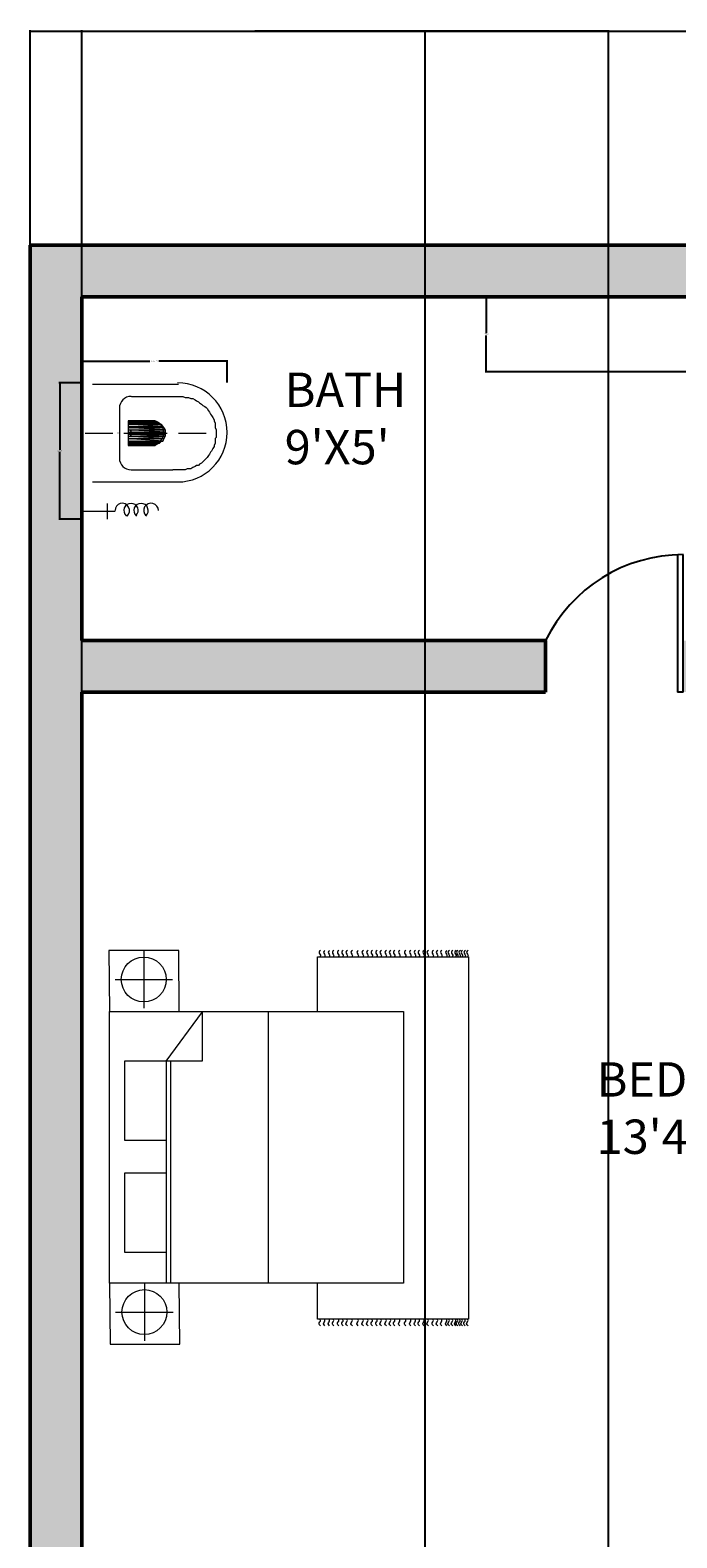
# Model space of a CAD drawing. Units: inches. Extents: x 383 to 970, y 275 to 1088.
# Tile 7 of 11: x 420 to 533, y 825 to 1088. Entities that reach past the tile are written whole.
import ezdxf

# ---------------------------------------------------------------- set-up
doc = ezdxf.new("R2010")
doc.units = ezdxf.units.IN
doc.header["$MEASUREMENT"] = 0
for name, color, linetype, lineweight in [('A-ANNO-DIMS', 2, 'Continuous', 18), ('A-AREA-IDEN', 7, 'Continuous', 18), ('A-DOOR', 3, 'Continuous', 25), ('A-FLOR-FIXT', 8, 'Continuous', 18), ('A-FURN', 8, 'Continuous', 18), ('A-WALL', 7, 'Continuous', 50)]:
    doc.layers.add(name, color=color, linetype=linetype, lineweight=lineweight)
doc.layers.add('A-WALL-PATT', color=251, linetype='Continuous', lineweight=13, true_color=0x636466)
doc.styles.get("Standard").update_dxf_attribs({"font": 'arial.ttf'})
doc.dimstyles.get("Standard").update_dxf_attribs({"dimtxt": 0.18, "dimasz": 0.18, "dimexe": 0.18, "dimexo": 0.0625, "dimgap": 0.09, "dimtad": 0, "dimtih": 1, "dimtoh": 1, "dimdec": 4, "dimzin": 0, "dimdsep": 46, "dimtxsty": 'Standard', "dimcen": 0.09, "dimadec": 0, "dimazin": 0, "dimtfac": 1, "dimtdec": 4, "dimtofl": 0, "dimtmove": 0, "dimatfit": 3, "dimfxl": 1, "dimtolj": 1, "dimtzin": 0, "dimarcsym": 0})

# ---------------------------------------------------------------- blocks, each defined once
blk = doc.blocks.new('BED-DOUBLE-WITH-NIGHTSTANDS')
for p, q in [((6.09, 68.68), (6.09, 58.62)), ((36.42, 67.59), (62.78, 67.59)), ((36.42, 58.05), (36.42, 67.59)), ((62.78, 67.59), (62.78, 4.35)), ((1.07, 63.65), (11.12, 63.65)), ((9.97, 49.39), (16.32, 58)), ((16.32, 49.44), (16.32, 58)), ((27.82, 58.05), (27.82, 10.63)), ((9.97, 49.44), (16.32, 49.44)), ((9.97, 49.39), (9.97, 10.63)), ((10.78, 49.44), (10.78, 10.63)), ((6.2, 10.63), (6.2, 0.57)), ((36.42, 4.35), (36.42, 10.65)), ((1.17, 5.6), (11.22, 5.6)), ((62.78, 4.35), (36.42, 4.35))]:
    blk.add_line(p, q)
for points in [[(12.29, 58.05), (12.19, 68.68), (0, 68.68), (0.1, 58.05)], [(0.1, 58.05), (51.42, 58.05), (51.42, 10.63), (0.1, 10.63)], [(2.8, 49.44), (9.97, 49.44), (9.97, 35.55), (2.8, 35.55)], [(2.8, 29.88), (9.97, 29.88), (9.97, 15.98), (2.8, 15.98)], [(12.39, 0), (12.29, 10.63), (0.1, 10.63), (0.21, 0)]]:
    blk.add_lwpolyline(points, close=True)
for centre in [(6.09, 63.65), (6.2, 5.6)]:
    blk.add_circle(centre, 3.92)
for points, knots in [([(36.95, 68.71), (36.83, 68.61), (36.59, 68.42), (36.83, 68.08), (37, 67.8), (36.89, 67.65), (36.85, 67.58)], [0, 0, 0, 0, 0.400747, 0.791423, 1.067667, 1.29709, 1.29709, 1.29709, 1.29709]), ([(37.73, 68.71), (37.61, 68.61), (37.37, 68.42), (37.61, 68.08), (37.78, 67.8), (37.67, 67.65), (37.62, 67.58)], [0, 0, 0, 0, 0.400747, 0.791423, 1.067667, 1.29709, 1.29709, 1.29709, 1.29709]), ([(38.54, 68.71), (38.42, 68.61), (38.18, 68.42), (38.42, 68.08), (38.59, 67.8), (38.49, 67.65), (38.44, 67.58)], [0, 0, 0, 0, 0.400747, 0.791423, 1.067667, 1.29709, 1.29709, 1.29709, 1.29709]), ([(39.27, 68.71), (39.15, 68.61), (38.91, 68.42), (39.15, 68.08), (39.32, 67.8), (39.22, 67.65), (39.17, 67.58)], [0, 0, 0, 0, 0.400747, 0.791423, 1.067667, 1.29709, 1.29709, 1.29709, 1.29709]), ([(40.15, 68.71), (40.03, 68.61), (39.79, 68.42), (40.03, 68.08), (40.21, 67.8), (40.1, 67.65), (40.05, 67.58)], [0, 0, 0, 0, 0.400747, 0.791423, 1.067667, 1.29709, 1.29709, 1.29709, 1.29709]), ([(40.91, 68.71), (40.78, 68.61), (40.54, 68.42), (40.78, 68.08), (40.96, 67.8), (40.85, 67.65), (40.8, 67.58)], [0, 0, 0, 0, 0.400747, 0.791423, 1.067667, 1.29709, 1.29709, 1.29709, 1.29709]), ([(41.63, 68.71), (41.51, 68.61), (41.27, 68.42), (41.51, 68.08), (41.69, 67.8), (41.58, 67.65), (41.53, 67.58)], [0, 0, 0, 0, 0.400747, 0.791423, 1.067667, 1.29709, 1.29709, 1.29709, 1.29709]), ([(42.52, 68.71), (42.39, 68.61), (42.16, 68.42), (42.39, 68.08), (42.57, 67.8), (42.46, 67.65), (42.41, 67.58)], [0, 0, 0, 0, 0.400747, 0.791423, 1.067667, 1.29709, 1.29709, 1.29709, 1.29709]), ([(43.55, 68.71), (43.43, 68.61), (43.19, 68.42), (43.43, 68.08), (43.6, 67.8), (43.5, 67.65), (43.45, 67.58)], [0, 0, 0, 0, 0.400747, 0.791423, 1.067667, 1.29709, 1.29709, 1.29709, 1.29709]), ([(44.43, 68.71), (44.31, 68.61), (44.07, 68.42), (44.31, 68.08), (44.49, 67.8), (44.38, 67.65), (44.33, 67.58)], [0, 0, 0, 0, 0.400747, 0.791423, 1.067667, 1.29709, 1.29709, 1.29709, 1.29709]), ([(45.25, 68.71), (45.13, 68.61), (44.89, 68.42), (45.13, 68.08), (45.3, 67.8), (45.2, 67.65), (45.15, 67.58)], [0, 0, 0, 0, 0.400747, 0.791423, 1.067667, 1.29709, 1.29709, 1.29709, 1.29709]), ([(46.03, 68.71), (45.91, 68.61), (45.67, 68.42), (45.91, 68.08), (46.08, 67.8), (45.97, 67.65), (45.92, 67.58)], [0, 0, 0, 0, 0.400747, 0.791423, 1.067667, 1.29709, 1.29709, 1.29709, 1.29709]), ([(46.84, 68.71), (46.72, 68.61), (46.48, 68.42), (46.72, 68.08), (46.9, 67.8), (46.79, 67.65), (46.74, 67.58)], [0, 0, 0, 0, 0.400747, 0.791423, 1.067667, 1.29709, 1.29709, 1.29709, 1.29709]), ([(47.57, 68.71), (47.45, 68.61), (47.21, 68.42), (47.45, 68.08), (47.62, 67.8), (47.52, 67.65), (47.47, 67.58)], [0, 0, 0, 0, 0.400747, 0.791423, 1.067667, 1.29709, 1.29709, 1.29709, 1.29709]), ([(48.45, 68.71), (48.33, 68.61), (48.09, 68.42), (48.33, 68.08), (48.51, 67.8), (48.4, 67.65), (48.35, 67.58)], [0, 0, 0, 0, 0.400747, 0.791423, 1.067667, 1.29709, 1.29709, 1.29709, 1.29709]), ([(49.21, 68.71), (49.08, 68.61), (48.85, 68.42), (49.08, 68.08), (49.26, 67.8), (49.15, 67.65), (49.1, 67.58)], [0, 0, 0, 0, 0.400747, 0.791423, 1.067667, 1.29709, 1.29709, 1.29709, 1.29709]), ([(49.93, 68.71), (49.81, 68.61), (49.57, 68.42), (49.81, 68.08), (49.99, 67.8), (49.88, 67.65), (49.83, 67.58)], [0, 0, 0, 0, 0.400747, 0.791423, 1.067667, 1.29709, 1.29709, 1.29709, 1.29709]), ([(50.82, 68.71), (50.69, 68.61), (50.46, 68.42), (50.69, 68.08), (50.87, 67.8), (50.76, 67.65), (50.71, 67.58)], [0, 0, 0, 0, 0.400747, 0.791423, 1.067667, 1.29709, 1.29709, 1.29709, 1.29709]), ([(51.85, 68.71), (51.73, 68.61), (51.49, 68.42), (51.73, 68.08), (51.9, 67.8), (51.8, 67.65), (51.75, 67.58)], [0, 0, 0, 0, 0.400747, 0.791423, 1.067667, 1.29709, 1.29709, 1.29709, 1.29709]), ([(52.74, 68.71), (52.61, 68.61), (52.37, 68.42), (52.61, 68.08), (52.79, 67.8), (52.68, 67.65), (52.63, 67.58)], [0, 0, 0, 0, 0.400747, 0.791423, 1.067667, 1.29709, 1.29709, 1.29709, 1.29709]), ([(53.55, 68.71), (53.43, 68.61), (53.19, 68.42), (53.43, 68.08), (53.6, 67.8), (53.5, 67.65), (53.45, 67.58)], [0, 0, 0, 0, 0.400747, 0.791423, 1.067667, 1.29709, 1.29709, 1.29709, 1.29709]), ([(54.24, 68.71), (54.12, 68.61), (53.88, 68.42), (54.12, 68.08), (54.29, 67.8), (54.19, 67.65), (54.14, 67.58)], [0, 0, 0, 0, 0.400747, 0.791423, 1.067667, 1.29709, 1.29709, 1.29709, 1.29709]), ([(55.06, 68.71), (54.94, 68.61), (54.7, 68.42), (54.94, 68.08), (55.11, 67.8), (55, 67.65), (54.95, 67.58)], [0, 0, 0, 0, 0.400747, 0.791423, 1.067667, 1.29709, 1.29709, 1.29709, 1.29709]), ([(55.78, 68.71), (55.66, 68.61), (55.42, 68.42), (55.66, 68.08), (55.84, 67.8), (55.73, 67.65), (55.68, 67.58)], [0, 0, 0, 0, 0.400747, 0.791423, 1.067667, 1.29709, 1.29709, 1.29709, 1.29709]), ([(56.67, 68.71), (56.55, 68.61), (56.31, 68.42), (56.55, 68.08), (56.72, 67.8), (56.61, 67.65), (56.56, 67.58)], [0, 0, 0, 0, 0.400747, 0.791423, 1.067667, 1.29709, 1.29709, 1.29709, 1.29709]), ([(57.42, 68.71), (57.3, 68.61), (57.06, 68.42), (57.3, 68.08), (57.47, 67.8), (57.36, 67.65), (57.32, 67.58)], [0, 0, 0, 0, 0.400747, 0.791423, 1.067667, 1.29709, 1.29709, 1.29709, 1.29709]), ([(58.15, 68.71), (58.03, 68.61), (57.79, 68.42), (58.03, 68.08), (58.2, 67.8), (58.1, 67.66), (58.05, 67.59)], [0, 0, 0, 0, 0.400747, 0.791423, 1.067667, 1.283686, 1.283686, 1.283686, 1.283686]), ([(59.03, 68.71), (58.91, 68.61), (58.67, 68.42), (58.91, 68.08), (59.08, 67.8), (58.98, 67.66), (58.93, 67.59)], [0, 0, 0, 0, 0.400747, 0.791423, 1.067667, 1.283686, 1.283686, 1.283686, 1.283686]), ([(59.46, 68.71), (59.34, 68.61), (59.09, 68.42), (59.34, 68.08), (59.51, 67.8), (59.41, 67.66), (59.36, 67.59)], [0, 0, 0, 0, 0.402903, 0.794912, 1.071156, 1.287177, 1.287177, 1.287177, 1.287177]), ([(60.05, 68.71), (59.93, 68.61), (59.69, 68.42), (59.93, 68.08), (60.1, 67.8), (60, 67.66), (59.96, 67.59)], [0, 0, 0, 0, 0.400747, 0.791423, 1.067667, 1.283686, 1.283686, 1.283686, 1.283686]), ([(60.63, 68.71), (60.51, 68.61), (60.27, 68.42), (60.51, 68.08), (60.68, 67.8), (60.58, 67.66), (60.53, 67.59)], [0, 0, 0, 0, 0.400747, 0.791423, 1.067667, 1.283686, 1.283686, 1.283686, 1.283686]), ([(60.94, 68.71), (60.82, 68.61), (60.58, 68.42), (60.81, 68.08), (60.99, 67.8), (60.89, 67.66), (60.84, 67.59)], [0, 0, 0, 0, 0.400747, 0.791423, 1.067667, 1.283686, 1.283686, 1.283686, 1.283686]), ([(61.36, 68.71), (61.23, 68.61), (60.99, 68.42), (61.23, 68.08), (61.41, 67.8), (61.3, 67.65), (61.25, 67.58)], [0, 0, 0, 0, 0.400747, 0.791423, 1.067667, 1.29709, 1.29709, 1.29709, 1.29709]), ([(61.75, 68.71), (61.63, 68.61), (61.39, 68.42), (61.63, 68.08), (61.8, 67.8), (61.7, 67.65), (61.65, 67.58)], [0, 0, 0, 0, 0.400747, 0.791423, 1.067667, 1.29709, 1.29709, 1.29709, 1.29709]), ([(62.24, 68.71), (62.12, 68.61), (61.88, 68.42), (62.12, 68.08), (62.29, 67.8), (62.18, 67.65), (62.13, 67.58)], [0, 0, 0, 0, 0.400747, 0.791423, 1.067667, 1.29709, 1.29709, 1.29709, 1.29709]), ([(62.71, 68.71), (62.59, 68.61), (62.35, 68.42), (62.59, 68.08), (62.76, 67.8), (62.66, 67.65), (62.61, 67.58)], [0, 0, 0, 0, 0.400747, 0.791423, 1.067667, 1.29709, 1.29709, 1.29709, 1.29709]), ([(36.95, 3.23), (36.83, 3.32), (36.59, 3.52), (36.83, 3.86), (37, 4.14), (36.89, 4.29), (36.85, 4.35)], [0, 0, 0, 0, 0.400747, 0.791423, 1.067667, 1.29709, 1.29709, 1.29709, 1.29709]), ([(37.73, 3.23), (37.61, 3.32), (37.37, 3.52), (37.61, 3.86), (37.78, 4.14), (37.67, 4.29), (37.62, 4.35)], [0, 0, 0, 0, 0.400747, 0.791423, 1.067667, 1.29709, 1.29709, 1.29709, 1.29709]), ([(38.54, 3.23), (38.42, 3.32), (38.18, 3.52), (38.42, 3.86), (38.59, 4.14), (38.49, 4.29), (38.44, 4.35)], [0, 0, 0, 0, 0.400747, 0.791423, 1.067667, 1.29709, 1.29709, 1.29709, 1.29709]), ([(39.27, 3.23), (39.15, 3.32), (38.91, 3.52), (39.15, 3.86), (39.32, 4.14), (39.22, 4.29), (39.17, 4.35)], [0, 0, 0, 0, 0.400747, 0.791423, 1.067667, 1.29709, 1.29709, 1.29709, 1.29709]), ([(40.15, 3.23), (40.03, 3.32), (39.79, 3.52), (40.03, 3.86), (40.21, 4.14), (40.1, 4.29), (40.05, 4.35)], [0, 0, 0, 0, 0.400747, 0.791423, 1.067667, 1.29709, 1.29709, 1.29709, 1.29709]), ([(40.91, 3.23), (40.78, 3.32), (40.54, 3.52), (40.78, 3.86), (40.96, 4.14), (40.85, 4.29), (40.8, 4.35)], [0, 0, 0, 0, 0.400747, 0.791423, 1.067667, 1.29709, 1.29709, 1.29709, 1.29709]), ([(41.63, 3.23), (41.51, 3.32), (41.27, 3.52), (41.51, 3.86), (41.69, 4.14), (41.58, 4.29), (41.53, 4.35)], [0, 0, 0, 0, 0.400747, 0.791423, 1.067667, 1.29709, 1.29709, 1.29709, 1.29709]), ([(42.52, 3.23), (42.39, 3.32), (42.16, 3.52), (42.39, 3.86), (42.57, 4.14), (42.46, 4.29), (42.41, 4.35)], [0, 0, 0, 0, 0.400747, 0.791423, 1.067667, 1.29709, 1.29709, 1.29709, 1.29709]), ([(43.55, 3.23), (43.43, 3.32), (43.19, 3.52), (43.43, 3.86), (43.6, 4.14), (43.5, 4.29), (43.45, 4.35)], [0, 0, 0, 0, 0.400747, 0.791423, 1.067667, 1.29709, 1.29709, 1.29709, 1.29709]), ([(44.43, 3.23), (44.31, 3.32), (44.07, 3.52), (44.31, 3.86), (44.49, 4.14), (44.38, 4.29), (44.33, 4.35)], [0, 0, 0, 0, 0.400747, 0.791423, 1.067667, 1.29709, 1.29709, 1.29709, 1.29709]), ([(45.25, 3.23), (45.13, 3.32), (44.89, 3.52), (45.13, 3.86), (45.3, 4.14), (45.2, 4.29), (45.15, 4.35)], [0, 0, 0, 0, 0.400747, 0.791423, 1.067667, 1.29709, 1.29709, 1.29709, 1.29709]), ([(46.03, 3.23), (45.91, 3.32), (45.67, 3.52), (45.91, 3.86), (46.08, 4.14), (45.97, 4.29), (45.92, 4.35)], [0, 0, 0, 0, 0.400747, 0.791423, 1.067667, 1.29709, 1.29709, 1.29709, 1.29709]), ([(46.84, 3.23), (46.72, 3.32), (46.48, 3.52), (46.72, 3.86), (46.9, 4.14), (46.79, 4.29), (46.74, 4.35)], [0, 0, 0, 0, 0.400747, 0.791423, 1.067667, 1.29709, 1.29709, 1.29709, 1.29709]), ([(47.57, 3.23), (47.45, 3.32), (47.21, 3.52), (47.45, 3.86), (47.62, 4.14), (47.52, 4.29), (47.47, 4.35)], [0, 0, 0, 0, 0.400747, 0.791423, 1.067667, 1.29709, 1.29709, 1.29709, 1.29709]), ([(48.45, 3.23), (48.33, 3.32), (48.09, 3.52), (48.33, 3.86), (48.51, 4.14), (48.4, 4.29), (48.35, 4.35)], [0, 0, 0, 0, 0.400747, 0.791423, 1.067667, 1.29709, 1.29709, 1.29709, 1.29709]), ([(49.21, 3.23), (49.08, 3.32), (48.85, 3.52), (49.08, 3.86), (49.26, 4.14), (49.15, 4.29), (49.1, 4.35)], [0, 0, 0, 0, 0.400747, 0.791423, 1.067667, 1.29709, 1.29709, 1.29709, 1.29709]), ([(49.93, 3.23), (49.81, 3.32), (49.57, 3.52), (49.81, 3.86), (49.99, 4.14), (49.88, 4.29), (49.83, 4.35)], [0, 0, 0, 0, 0.400747, 0.791423, 1.067667, 1.29709, 1.29709, 1.29709, 1.29709]), ([(50.82, 3.23), (50.69, 3.32), (50.46, 3.52), (50.69, 3.86), (50.87, 4.14), (50.76, 4.29), (50.71, 4.35)], [0, 0, 0, 0, 0.400747, 0.791423, 1.067667, 1.29709, 1.29709, 1.29709, 1.29709]), ([(51.85, 3.23), (51.73, 3.32), (51.49, 3.52), (51.73, 3.86), (51.9, 4.14), (51.8, 4.29), (51.75, 4.35)], [0, 0, 0, 0, 0.400747, 0.791423, 1.067667, 1.29709, 1.29709, 1.29709, 1.29709]), ([(52.74, 3.23), (52.61, 3.32), (52.37, 3.52), (52.61, 3.86), (52.79, 4.14), (52.68, 4.29), (52.63, 4.35)], [0, 0, 0, 0, 0.400747, 0.791423, 1.067667, 1.29709, 1.29709, 1.29709, 1.29709]), ([(53.55, 3.23), (53.43, 3.32), (53.19, 3.52), (53.43, 3.86), (53.6, 4.14), (53.5, 4.29), (53.45, 4.35)], [0, 0, 0, 0, 0.400747, 0.791423, 1.067667, 1.29709, 1.29709, 1.29709, 1.29709]), ([(54.24, 3.23), (54.12, 3.32), (53.88, 3.52), (54.12, 3.86), (54.29, 4.14), (54.19, 4.29), (54.14, 4.35)], [0, 0, 0, 0, 0.400747, 0.791423, 1.067667, 1.29709, 1.29709, 1.29709, 1.29709]), ([(55.06, 3.23), (54.94, 3.32), (54.7, 3.52), (54.94, 3.86), (55.11, 4.14), (55, 4.29), (54.95, 4.35)], [0, 0, 0, 0, 0.400747, 0.791423, 1.067667, 1.29709, 1.29709, 1.29709, 1.29709]), ([(55.78, 3.23), (55.66, 3.32), (55.42, 3.52), (55.66, 3.86), (55.84, 4.14), (55.73, 4.29), (55.68, 4.35)], [0, 0, 0, 0, 0.400747, 0.791423, 1.067667, 1.29709, 1.29709, 1.29709, 1.29709]), ([(56.67, 3.23), (56.55, 3.32), (56.31, 3.52), (56.55, 3.86), (56.72, 4.14), (56.61, 4.29), (56.56, 4.35)], [0, 0, 0, 0, 0.400747, 0.791423, 1.067667, 1.29709, 1.29709, 1.29709, 1.29709]), ([(57.42, 3.23), (57.3, 3.32), (57.06, 3.52), (57.3, 3.86), (57.47, 4.14), (57.36, 4.29), (57.32, 4.35)], [0, 0, 0, 0, 0.400747, 0.791423, 1.067667, 1.29709, 1.29709, 1.29709, 1.29709]), ([(58.15, 3.23), (58.03, 3.32), (57.79, 3.52), (58.03, 3.86), (58.2, 4.14), (58.09, 4.29), (58.04, 4.35)], [0, 0, 0, 0, 0.400747, 0.791423, 1.067667, 1.29709, 1.29709, 1.29709, 1.29709]), ([(59.03, 3.23), (58.91, 3.32), (58.67, 3.52), (58.91, 3.86), (59.08, 4.14), (58.98, 4.29), (58.93, 4.35)], [0, 0, 0, 0, 0.400747, 0.791423, 1.067667, 1.29709, 1.29709, 1.29709, 1.29709]), ([(59.46, 3.23), (59.33, 3.32), (59.08, 3.52), (59.34, 3.86), (59.51, 4.14), (59.4, 4.29), (59.36, 4.35)], [0, 0, 0, 0, 0.407265, 0.802015, 1.07826, 1.307683, 1.307683, 1.307683, 1.307683]), ([(60.03, 3.23), (59.9, 3.32), (59.67, 3.52), (59.9, 3.86), (60.08, 4.14), (59.97, 4.29), (59.92, 4.35)], [0, 0, 0, 0, 0.400747, 0.791423, 1.067667, 1.29709, 1.29709, 1.29709, 1.29709]), ([(60.6, 3.23), (60.48, 3.32), (60.24, 3.52), (60.48, 3.86), (60.65, 4.14), (60.54, 4.29), (60.5, 4.35)], [0, 0, 0, 0, 0.400747, 0.791423, 1.067667, 1.29709, 1.29709, 1.29709, 1.29709]), ([(60.91, 3.23), (60.79, 3.32), (60.55, 3.52), (60.79, 3.86), (60.96, 4.14), (60.85, 4.29), (60.81, 4.35)], [0, 0, 0, 0, 0.400747, 0.791423, 1.067667, 1.29709, 1.29709, 1.29709, 1.29709]), ([(61.33, 3.23), (61.21, 3.32), (60.97, 3.52), (61.21, 3.86), (61.38, 4.14), (61.27, 4.29), (61.22, 4.35)], [0, 0, 0, 0, 0.400747, 0.791423, 1.067667, 1.29709, 1.29709, 1.29709, 1.29709]), ([(61.72, 3.23), (61.6, 3.32), (61.36, 3.52), (61.6, 3.86), (61.78, 4.14), (61.67, 4.29), (61.62, 4.35)], [0, 0, 0, 0, 0.400747, 0.791423, 1.067667, 1.29709, 1.29709, 1.29709, 1.29709]), ([(62.21, 3.23), (62.09, 3.32), (61.85, 3.52), (62.09, 3.86), (62.26, 4.14), (62.16, 4.29), (62.11, 4.35)], [0, 0, 0, 0, 0.400747, 0.791423, 1.067667, 1.29709, 1.29709, 1.29709, 1.29709]), ([(62.71, 3.23), (62.59, 3.32), (62.35, 3.52), (62.59, 3.86), (62.76, 4.14), (62.66, 4.29), (62.61, 4.35)], [0, 0, 0, 0, 0.400747, 0.791423, 1.067667, 1.29709, 1.29709, 1.29709, 1.29709])]:
    blk.add_open_spline(points, degree=3, knots=knots)
blk = doc.blocks.new('WC-PLAN')
h = blk.add_hatch(color=256)
h.paths.add_polyline_path([(8.12, 16.94), (13.2, 16.94), (8.12, 17.17)])
h.paths.add_polyline_path([(13.2, 16.94), (8.12, 17.17), (12.82, 17.17)])
h.paths.add_polyline_path([(8.12, 17.17), (12.82, 17.17), (12.44, 17.17)])
h = blk.add_hatch(color=256)
h.paths.add_polyline_path([(8.12, 16.71), (13.58, 16.71), (8.12, 16.94)])
h.paths.add_polyline_path([(13.58, 16.71), (8.12, 16.94), (13.2, 16.94)])
h = blk.add_hatch(color=256)
h.paths.add_polyline_path([(8.12, 16.56), (13.81, 16.56), (8.12, 16.71)])
h.paths.add_polyline_path([(13.81, 16.56), (8.12, 16.71), (13.58, 16.71)])
h = blk.add_hatch(color=256)
h.paths.add_polyline_path([(8.12, 16.18), (14.19, 16.18), (8.12, 16.56)])
h.paths.add_polyline_path([(14.19, 16.18), (8.12, 16.56), (13.81, 16.56)])
h = blk.add_hatch(color=256)
h.paths.add_polyline_path([(8.12, 15.95), (14.34, 15.95), (8.12, 16.18)])
h.paths.add_polyline_path([(14.34, 15.95), (8.12, 16.18), (14.19, 16.18)])
h = blk.add_hatch(color=256)
h.paths.add_polyline_path([(8.12, 15.57), (14.56, 15.57), (8.12, 15.95)])
h.paths.add_polyline_path([(14.56, 15.57), (8.12, 15.95), (14.34, 15.95)])
h = blk.add_hatch(color=256)
h.paths.add_polyline_path([(8.12, 15.19), (14.56, 15.19), (8.12, 15.57)])
h.paths.add_polyline_path([(14.56, 15.19), (8.12, 15.57), (14.56, 15.57)])
h = blk.add_hatch(color=256)
h.paths.add_polyline_path([(8.12, 14.81), (14.56, 14.81), (8.12, 15.19)])
h.paths.add_polyline_path([(14.56, 14.81), (8.12, 15.19), (14.56, 15.19)])
h = blk.add_hatch(color=256)
h.paths.add_polyline_path([(8.12, 14.44), (14.56, 14.44), (8.12, 14.81)])
h.paths.add_polyline_path([(14.56, 14.44), (8.12, 14.81), (14.56, 14.81)])
h = blk.add_hatch(color=256)
h.paths.add_polyline_path([(8.12, 14.06), (14.34, 14.06), (8.12, 14.44)])
h.paths.add_polyline_path([(14.34, 14.06), (8.12, 14.44), (14.56, 14.44)])
h = blk.add_hatch(color=256)
h.paths.add_polyline_path([(8.12, 13.6), (14.19, 13.6), (8.12, 14.06)])
h.paths.add_polyline_path([(14.19, 13.6), (8.12, 14.06), (14.34, 14.06)])
h = blk.add_hatch(color=256)
h.paths.add_polyline_path([(8.12, 13.45), (13.81, 13.45), (8.12, 13.6)])
h.paths.add_polyline_path([(13.81, 13.45), (8.12, 13.6), (14.19, 13.6)])
h = blk.add_hatch(color=256)
h.paths.add_polyline_path([(8.12, 13.22), (13.58, 13.22), (8.12, 13.45)])
h.paths.add_polyline_path([(13.58, 13.22), (8.12, 13.45), (13.81, 13.45)])
h = blk.add_hatch(color=256)
h.paths.add_polyline_path([(8.12, 13.07), (13.2, 13.07), (8.12, 13.22)])
h.paths.add_polyline_path([(13.2, 13.07), (8.12, 13.22), (13.58, 13.22)])
h = blk.add_hatch(color=256)
h.paths.add_polyline_path([(8.12, 12.84), (12.82, 12.84), (8.12, 13.07)])
h.paths.add_polyline_path([(12.82, 12.84), (8.12, 13.07), (13.2, 13.07)])
for points in [[(1.9, 23.54), (16.92, 23.54), (16.92, 23.54)], [(8.72, 21.41), (15.93, 21.41), (15.93, 21.41)], [(15.93, 21.41), (16.69, 21.41), (17.3, 21.41), (17.67, 21.41), (18.05, 21.19), (18.43, 21.19), (18.66, 21.19), (19.04, 21.03), (19.42, 21.03), (19.8, 20.81), (20.03, 20.66), (20.41, 20.43), (20.56, 20.28), (20.94, 20.05), (21.16, 19.82), (21.54, 19.67), (21.77, 19.44), (21.92, 19.29), (22.15, 18.91), (22.3, 18.68), (22.53, 18.3), (22.68, 18.08), (22.91, 17.7), (23.14, 17.32), (23.14, 17.17), (23.29, 16.71), (23.29, 16.33), (23.29, 15.95), (23.52, 15.57), (23.52, 14.97), (23.52, 14.21), (23.29, 14.06), (23.29, 13.6), (23.29, 13.22), (23.14, 12.84), (23.14, 12.69), (22.91, 12.31), (22.68, 11.86), (22.53, 11.7), (22.3, 11.32), (22.15, 11.1), (21.92, 10.72), (21.77, 10.57), (21.54, 10.34), (21.16, 9.96), (20.94, 9.73), (20.56, 9.58), (20.41, 9.35), (20.03, 9.35), (19.8, 9.2), (19.42, 8.97), (19.04, 8.75), (18.66, 8.75), (18.43, 8.75), (18.05, 8.59), (17.67, 8.59), (17.3, 8.59), (16.69, 8.59), (15.93, 8.59)], [(6.6, 19.29), (6.6, 10.57), (6.6, 10.57)], [(8.12, 17.17), (8.12, 12.84), (8.12, 12.84)], [(8.12, 17.17), (12.44, 17.17), (12.44, 17.17)], [(0.61, 14.97), (5.46, 14.97), (5.46, 14.97)], [(6.37, 14.97), (6.37, 15.04), (6.37, 15.04)], [(7.36, 14.97), (14.94, 14.97), (14.94, 14.97)], [(8.57, 15.42), (8.5, 15.42), (8.5, 15.42)], [(8.57, 14.97), (8.5, 15.04), (8.5, 15.04)], [(8.57, 14.59), (8.5, 14.59), (8.5, 14.59)], [(8.57, 15.42), (8.57, 15.19), (8.57, 14.97)], [(8.57, 14.97), (8.57, 14.81), (8.57, 14.59)], [(16.92, 14.97), (21.77, 14.97), (21.77, 14.97)], [(8.12, 12.84), (12.44, 12.84), (12.44, 12.84)], [(8.72, 8.59), (15.93, 8.59), (15.93, 8.59)], [(1.9, 6.47), (16.92, 6.47), (16.92, 6.47)], [(4.48, 2.73), (4.48, 0), (4.48, 0)], [(0, 1.37), (5.84, 1.37), (5.84, 1.37)]]:
    blk.add_lwpolyline(points)
for points in [[(8.12, 16.94), (13.2, 16.94), (8.12, 17.17)], [(13.2, 16.94), (8.12, 17.17), (12.82, 17.17)], [(8.12, 17.17), (12.82, 17.17), (12.44, 17.17)], [(12.82, 17.17), (8.12, 17.17), (8.12, 17.17)], [(8.12, 16.71), (13.58, 16.71), (8.12, 16.94)], [(13.58, 16.71), (8.12, 16.94), (13.2, 16.94)], [(8.12, 16.56), (13.81, 16.56), (8.12, 16.71)], [(13.81, 16.56), (8.12, 16.71), (13.58, 16.71)], [(8.12, 16.18), (14.19, 16.18), (8.12, 16.56)], [(14.19, 16.18), (8.12, 16.56), (13.81, 16.56)], [(8.12, 15.95), (14.34, 15.95), (8.12, 16.18)], [(14.34, 15.95), (8.12, 16.18), (14.19, 16.18)], [(8.12, 15.57), (14.56, 15.57), (8.12, 15.95)], [(14.56, 15.57), (8.12, 15.95), (14.34, 15.95)], [(8.12, 15.19), (14.56, 15.19), (8.12, 15.57)], [(14.56, 15.19), (8.12, 15.57), (14.56, 15.57)], [(8.12, 14.81), (14.56, 14.81), (8.12, 15.19)], [(14.56, 14.81), (8.12, 15.19), (14.56, 15.19)], [(8.12, 14.44), (14.56, 14.44), (8.12, 14.81)], [(14.56, 14.44), (8.12, 14.81), (14.56, 14.81)], [(8.12, 14.06), (14.34, 14.06), (8.12, 14.44)], [(14.34, 14.06), (8.12, 14.44), (14.56, 14.44)], [(8.12, 13.6), (14.19, 13.6), (8.12, 14.06)], [(14.19, 13.6), (8.12, 14.06), (14.34, 14.06)], [(8.12, 13.45), (13.81, 13.45), (8.12, 13.6)], [(13.81, 13.45), (8.12, 13.6), (14.19, 13.6)], [(8.12, 13.22), (13.58, 13.22), (8.12, 13.45)], [(13.58, 13.22), (8.12, 13.45), (13.81, 13.45)], [(8.12, 13.07), (13.2, 13.07), (8.12, 13.22)], [(13.2, 13.07), (8.12, 13.22), (13.58, 13.22)], [(8.12, 12.84), (12.82, 12.84), (8.12, 13.07)], [(12.82, 12.84), (8.12, 13.07), (13.2, 13.07)], [(8.12, 12.84), (12.44, 12.84)], [(12.44, 12.84), (8.12, 12.84), (12.82, 12.84)]]:
    blk.add_lwpolyline(points, close=True)
for points, knots in [([(16.76, 6.47), (21.54, 6.47), (25.41, 10.34), (25.41, 15.12), (25.41, 15.12), (25.41, 19.9), (21.54, 23.77), (16.76, 23.77)], [0, 0, 0, 0, 0.125, 0.125, 0.125, 0.125001, 1, 1, 1, 1]), ([(12.29, 13.07), (13.43, 13.07), (14.34, 13.98), (14.34, 15.12), (14.34, 15.12), (14.34, 16.26), (13.43, 17.17), (12.29, 17.17)], [0, 0, 0, 0, 0.125, 0.125, 0.125, 0.125001, 1, 1, 1, 1]), ([(7.97, 0.53), (8.34, 0.91), (8.5, 1.59), (8.19, 2.05), (8.19, 2.05), (7.89, 2.58), (7.36, 2.88), (6.75, 2.73), (6.75, 2.73), (6.22, 2.58), (5.84, 2.05), (5.84, 1.52)], [0, 0, 0, 0, 0.083333, 0.083333, 0.083333, 0.083334, 0.166667, 0.166667, 0.166667, 0.166668, 1, 1, 1, 1]), ([(9.48, 0.61), (9.86, 0.91), (10.01, 1.52), (9.79, 1.97), (9.79, 1.97), (9.63, 2.43), (9.1, 2.73), (8.65, 2.73), (8.65, 2.73), (8.12, 2.73), (7.66, 2.43), (7.43, 1.97), (7.43, 1.97), (7.28, 1.44), (7.43, 0.91), (7.81, 0.53)], [0, 0, 0, 0, 0.0625, 0.0625, 0.0625, 0.062501, 0.125, 0.125, 0.125, 0.125001, 0.1875, 0.1875, 0.1875, 0.187501, 1, 1, 1, 1]), ([(11.23, 0.53), (11.61, 0.91), (11.76, 1.44), (11.53, 1.97), (11.53, 1.97), (11.38, 2.43), (10.92, 2.73), (10.39, 2.73), (10.39, 2.73), (9.86, 2.73), (9.41, 2.43), (9.18, 1.97), (9.18, 1.97), (9.03, 1.44), (9.18, 0.91), (9.56, 0.53)], [0, 0, 0, 0, 0.0625, 0.0625, 0.0625, 0.062501, 0.125, 0.125, 0.125, 0.125001, 0.1875, 0.1875, 0.1875, 0.187501, 1, 1, 1, 1]), ([(13.43, 1.52), (13.43, 2.05), (12.97, 2.58), (12.44, 2.73), (12.44, 2.73), (11.91, 2.88), (11.3, 2.58), (11, 2.12), (11, 2.12), (10.77, 1.59), (10.85, 0.99), (11.23, 0.61)], [0, 0, 0, 0, 0.083333, 0.083333, 0.083333, 0.083334, 0.166667, 0.166667, 0.166667, 0.166668, 1, 1, 1, 1])]:
    blk.add_open_spline(points, degree=3, knots=knots)
for points in [[(8.65, 21.41), (7.51, 21.41), (6.6, 20.5), (6.6, 19.37)], [(6.6, 10.64), (6.6, 9.5), (7.51, 8.59), (8.65, 8.59)]]:
    blk.add_open_spline(points, degree=3)
blk = doc.blocks.new('DOOR-LEAF-24IN')
for p, q in [((23, 24), (23, 0)), ((24, 0), (24, 24)), ((24, 0), (23, 0))]:
    blk.add_line(p, q)
blk.add_arc((24, -2.7), 26.7, 90, 154.0108)
blk = doc.blocks.new('*D27')
at = {"layer": 'A-ANNO-DIMS', "color": 0, "lineweight": -2, "transparency": 16777216}
for p, q in [((429.23, 1026.17), (429.23, 1030.1)), ((429.41, 1029.92), (441.16, 1029.92)), ((454.46, 1029.92), (442.71, 1029.92)), ((454.64, 1026.17), (454.64, 1030.1))]:
    blk.add_line(p, q, dxfattribs=at)
at = {"layer": 'A-ANNO-DIMS', "color": 0, "transparency": 16777216}
for points in [[(429.41, 1029.95), (429.41, 1029.89), (429.23, 1029.92)], [(454.46, 1029.95), (454.46, 1029.89), (454.64, 1029.92)]]:
    blk.add_solid(points, dxfattribs=at)
at = {"layer": 'Defpoints', "color": 0, "transparency": 16777216}
for p in [(454.64, 1029.92), (429.23, 1026.11), (454.64, 1026.11)]:
    blk.add_point(p, dxfattribs=at)
at = {"layer": 'A-ANNO-DIMS', "color": 0, "transparency": 16777216, "insert": (441.94, 1029.92), "char_height": 0.18, "attachment_point": 5}
blk.add_mtext('\\A1;WC 25 TYP.', dxfattribs=at)
blk = doc.blocks.new('*D28')
at = {"layer": 'A-ANNO-DIMS', "color": 0, "lineweight": -2, "transparency": 16777216}
for p, q in [((429.17, 1026.11), (425.24, 1026.11)), ((425.42, 1025.93), (425.42, 1014.41)), ((425.42, 1002.53), (425.42, 1014.05)), ((429.17, 1002.35), (425.24, 1002.35))]:
    blk.add_line(p, q, dxfattribs=at)
at = {"layer": 'A-ANNO-DIMS', "color": 0, "transparency": 16777216}
for points in [[(425.39, 1025.93), (425.45, 1025.93), (425.42, 1026.11)], [(425.39, 1002.53), (425.45, 1002.53), (425.42, 1002.35)]]:
    blk.add_solid(points, dxfattribs=at)
at = {"layer": 'Defpoints', "color": 0, "transparency": 16777216}
for p in [(425.42, 1026.11), (429.23, 1026.11), (429.23, 1002.35)]:
    blk.add_point(p, dxfattribs=at)
at = {"layer": 'A-ANNO-DIMS', "color": 0, "transparency": 16777216, "insert": (425.42, 1014.23), "char_height": 0.18, "attachment_point": 5}
blk.add_mtext('\\A1;24 TYP.', dxfattribs=at)
blk = doc.blocks.new('*D37')
at = {"layer": 'A-ANNO-DIMS', "color": 0, "lineweight": -2, "transparency": 16777216}
for p, q in [((420.24, 1050.2), (420.24, 1087.67)), ((420.42, 1087.49), (675.95, 1087.49)), ((932.06, 1087.49), (676.53, 1087.49)), ((932.24, 1050.2), (932.24, 1087.67))]:
    blk.add_line(p, q, dxfattribs=at)
at = {"layer": 'A-ANNO-DIMS', "color": 0, "transparency": 16777216}
for points in [[(420.42, 1087.52), (420.42, 1087.46), (420.24, 1087.49)], [(932.06, 1087.52), (932.06, 1087.46), (932.24, 1087.49)]]:
    blk.add_solid(points, dxfattribs=at)
at = {"layer": 'Defpoints', "color": 0, "transparency": 16777216}
for p in [(932.24, 1087.49), (420.24, 1050.14), (932.24, 1050.14)]:
    blk.add_point(p, dxfattribs=at)
at = {"layer": 'A-ANNO-DIMS', "color": 0, "transparency": 16777216, "insert": (676.24, 1087.49), "char_height": 0.18, "attachment_point": 5}
blk.add_mtext('\\A1;512', dxfattribs=at)
blk = doc.blocks.new('*D48')
at = {"layer": 'A-ANNO-DIMS', "color": 0, "lineweight": -2, "transparency": 16777216}
for p, q in [((429.24, 546.2), (429.24, 1087.67)), ((429.42, 1087.49), (475.02, 1087.49)), ((521.06, 1087.49), (475.46, 1087.49)), ((521.24, 546.2), (521.24, 1087.67))]:
    blk.add_line(p, q, dxfattribs=at)
at = {"layer": 'A-ANNO-DIMS', "color": 0, "transparency": 16777216}
for points in [[(429.42, 1087.52), (429.42, 1087.46), (429.24, 1087.49)], [(521.06, 1087.52), (521.06, 1087.46), (521.24, 1087.49)]]:
    blk.add_solid(points, dxfattribs=at)
at = {"layer": 'Defpoints', "color": 0, "transparency": 16777216}
for p in [(521.24, 1087.49), (429.24, 546.14), (521.24, 546.14)]:
    blk.add_point(p, dxfattribs=at)
at = {"layer": 'A-ANNO-DIMS', "color": 0, "transparency": 16777216, "insert": (475.24, 1087.49), "char_height": 0.18, "attachment_point": 5}
blk.add_mtext('\\A1;92', dxfattribs=at)
blk = doc.blocks.new('*D49')
at = {"layer": 'A-ANNO-DIMS', "color": 0, "lineweight": -2, "transparency": 16777216}
for p, q in [((429.24, 615.2), (429.24, 1087.67)), ((429.42, 1087.49), (459.02, 1087.49)), ((489.06, 1087.49), (459.46, 1087.49)), ((489.24, 615.2), (489.24, 1087.67))]:
    blk.add_line(p, q, dxfattribs=at)
at = {"layer": 'A-ANNO-DIMS', "color": 0, "transparency": 16777216}
for points in [[(429.42, 1087.52), (429.42, 1087.46), (429.24, 1087.49)], [(489.06, 1087.52), (489.06, 1087.46), (489.24, 1087.49)]]:
    blk.add_solid(points, dxfattribs=at)
at = {"layer": 'Defpoints', "color": 0, "transparency": 16777216}
for p in [(489.24, 1087.49), (429.24, 615.14), (489.24, 615.14)]:
    blk.add_point(p, dxfattribs=at)
at = {"layer": 'A-ANNO-DIMS', "color": 0, "transparency": 16777216, "insert": (459.24, 1087.49), "char_height": 0.18, "attachment_point": 5}
blk.add_mtext('\\A1;60', dxfattribs=at)
blk = doc.blocks.new('*D62')
at = {"layer": 'A-ANNO-DIMS', "color": 0, "lineweight": -2, "transparency": 16777216}
for p, q in [((537.18, 1041.14), (499.71, 1041.14)), ((499.89, 1040.96), (499.89, 1034.77)), ((499.89, 1028.21), (499.89, 1034.4)), ((537.18, 1028.03), (499.71, 1028.03))]:
    blk.add_line(p, q, dxfattribs=at)
at = {"layer": 'A-ANNO-DIMS', "color": 0, "transparency": 16777216}
for points in [[(499.86, 1040.96), (499.92, 1040.96), (499.89, 1041.14)], [(499.86, 1028.21), (499.92, 1028.21), (499.89, 1028.03)]]:
    blk.add_solid(points, dxfattribs=at)
at = {"layer": 'Defpoints', "color": 0, "transparency": 16777216}
for p in [(499.89, 1041.14), (537.24, 1041.14), (537.24, 1028.03)]:
    blk.add_point(p, dxfattribs=at)
at = {"layer": 'A-ANNO-DIMS', "color": 0, "transparency": 16777216, "insert": (499.89, 1034.59), "char_height": 0.18, "attachment_point": 5}
blk.add_mtext('\\A1;13.103', dxfattribs=at)

msp = doc.modelspace()

# ---------------------------------------------------------------- hatches: boundary and pattern name
at = {"layer": 'A-WALL-PATT'}
h = msp.add_hatch(color=256, dxfattribs=at)
h.dxf.hatch_style = 1
h.paths.add_polyline_path([(651.24, 321.1365), (651.24, 417.1365), (735.24, 417.1365), (735.24, 491.9233), (726.24, 491.9233), (726.24, 426.1365), (582.24, 426.1365), (582.24, 606.1365), (687.24, 606.1365), (687.24, 615.1365), (573.24, 615.1365), (573.24, 546.1365), (570.24, 546.1365), (570.24, 537.1365), (573.24, 537.1365), (573.24, 414.1365), (582.24, 414.1365), (582.24, 417.1365), (642.24, 417.1365), (642.24, 321.1365), (621.6203, 321.1365), (621.6203, 312.1365), (651.24, 312.1365)], flags=17)
h.paths.add_polyline_path([(597.6203, 321.1365), (582.24, 321.1365), (582.24, 390.1365), (573.24, 390.1365), (573.24, 321.1365), (570.24, 321.1365), (570.24, 312.1365), (573.24, 312.1365), (597.6203, 312.1365)], flags=16)
h.paths.add_polyline_path([(534.24, 321.1365), (500.8868, 321.1365), (500.8868, 312.1365), (534.24, 312.1365)], flags=17)
h.paths.add_polyline_path([(735.24, 606.1365), (738.24, 606.1365), (738.24, 615.1365), (723.24, 615.1365), (723.24, 606.1365), (726.24, 606.1365), (726.24, 551.9233), (735.24, 551.9233)], flags=17)
h.paths.add_polyline_path([(848.0899, 615.1365), (814.24, 615.1365), (814.24, 689.38), (805.24, 689.38), (805.24, 615.1365), (802.24, 615.1365), (802.24, 606.1365), (848.0899, 606.1365)], flags=17)
h.paths.add_polyline_path([(530.24, 615.1365), (498.24, 615.1365), (498.24, 646.5351), (489.24, 646.5351), (489.24, 615.1365), (466.771, 615.1365), (466.771, 606.1365), (521.24, 606.1365), (521.24, 603.1365), (530.24, 603.1365), (530.24, 606.1365)], flags=17)
h.paths.add_polyline_path([(498.24, 744.1365), (489.24, 744.1365), (489.24, 706.5351), (498.24, 706.5351)], flags=17)
h.paths.add_polyline_path([(715.24, 792.1365), (598.24, 792.1365), (598.24, 972.1365), (636.5058, 972.1365), (636.5058, 981.1365), (589.24, 981.1365), (589.24, 972.1365), (589.24, 792.1365), (586.24, 792.1365), (586.24, 783.1365), (589.24, 783.1365), (715.24, 783.1365)], flags=17)
h.paths.add_polyline_path([(763.24, 981.1365), (696.5058, 981.1365), (696.5058, 972.1365), (754.24, 972.1365), (754.24, 792.1365), (751.24, 792.1365), (751.24, 783.1365), (754.24, 783.1365), (764.24, 783.1365), (764.24, 792.1365), (763.24, 792.1365)], flags=17)
h.paths.add_polyline_path([(815.24, 1001.9492), (806.24, 1001.9492), (806.24, 972.1365), (818.24, 972.1365), (818.24, 981.1365), (815.24, 981.1365)], flags=17)
h.paths.add_polyline_path([(546.24, 1004.0336), (537.24, 1004.0336), (537.24, 981.1365), (534.24, 981.1365), (534.24, 972.1365), (537.24, 972.1365), (546.24, 972.1365), (546.24, 981.1365)], flags=17)
h.paths.add_polyline_path([(884.0899, 606.1365), (932.24, 606.1365), (932.24, 1050.1365), (420.24, 1050.1365), (420.24, 312.1365), (440.8868, 312.1365), (440.8868, 321.1365), (429.24, 321.1365), (429.24, 537.1365), (538.24, 537.1365), (538.24, 546.1365), (530.24, 546.1365), (530.24, 579.1365), (521.24, 579.1365), (521.24, 546.1365), (429.24, 546.1365), (429.24, 606.1365), (442.771, 606.1365), (442.771, 615.1365), (429.24, 615.1365), (429.24, 783.1365), (489.24, 783.1365), (489.24, 780.1365), (498.24, 780.1365), (498.24, 783.1365), (550.24, 783.1365), (550.24, 792.1365), (429.24, 792.1365), (429.24, 972.1365), (510.24, 972.1365), (510.24, 981.1365), (429.24, 981.1365), (429.24, 1041.1365), (537.24, 1041.1365), (537.24, 1028.0336), (546.24, 1028.0336), (546.24, 1041.1365), (806.24, 1041.1365), (806.24, 1025.9492), (815.24, 1025.9492), (815.24, 1041.1365), (923.24, 1041.1365), (923.24, 981.1365), (842.24, 981.1365), (842.24, 972.1365), (923.24, 972.1365), (923.24, 792.1365), (800.24, 792.1365), (800.24, 783.1365), (805.24, 783.1365), (805.24, 725.38), (814.24, 725.38), (814.24, 783.1365), (923.24, 783.1365), (923.24, 615.1365), (884.0899, 615.1365)])

# ---------------------------------------------------------------- linework, layer by layer
at = {"layer": 'A-WALL'}
for p, q in [((420.24, 1050.1365), (932.24, 1050.1365)), ((420.24, 1050.1365), (420.24, 312.1365)), ((429.24, 1041.1365), (429.24, 981.1365)), ((429.24, 1041.1365), (537.24, 1041.1365)), ((429.24, 981.1365), (510.24, 981.1365)), ((510.24, 972.1365), (510.24, 981.1365)), ((429.24, 972.1365), (510.24, 972.1365)), ((429.24, 972.1365), (429.24, 792.1365))]:
    msp.add_line(p, q, dxfattribs=at)

# ---------------------------------------------------------------- block references
at = {"layer": 'A-DOOR'}
msp.add_blockref('DOOR-LEAF-24IN', (510.24, 972.136), dxfattribs=at)
at = {"layer": 'A-FLOR-FIXT'}
msp.add_blockref('WC-PLAN', (429.2289, 1002.3455), dxfattribs=at)
at = {"layer": 'A-FURN'}
msp.add_blockref('BED-DOUBLE-WITH-NIGHTSTANDS', (433.992, 858.347), dxfattribs=at)

# ---------------------------------------------------------------- texts
at = {"layer": 'A-AREA-IDEN', "char_height": 6, "attachment_point": 1}
for s, width, insert in [("BATH\\P9'X5'", 46.963316, (464.684, 1027.906)), ('BED ROOM\\P13\'4"X15\'0"', 49.692666, (519.1519, 907.5544))]:
    msp.add_mtext_dynamic_manual_height_columns(s, width=width, gutter_width=30, heights=[0], dxfattribs=dict(at, insert=insert))

# ---------------------------------------------------------------- dimensions: what is measured, and where the dimension line sits
at = {"layer": 'A-ANNO-DIMS'}
for base, p1, p2, picture, middle in [((932.24, 1087.4865), (420.24, 1050.1365), (932.24, 1050.1365), '*D37', (676.24, 1087.4865)), ((521.24, 1087.4865), (429.24, 546.1365), (521.24, 546.1365), '*D48', (475.24, 1087.4865)), ((489.24, 1087.4865), (429.24, 615.1365), (489.24, 615.1365), '*D49', (459.24, 1087.4865))]:
    dim = msp.add_linear_dim(base=base, p1=p1, p2=p2, dimstyle='Standard', override={"dimdec": 0, "dimlfac": 1, "dimrnd": 0, "dimzin": 0, "dimdsep": 46, "dimlunit": 2}, dxfattribs=at)
    dim.commit()
    dim.dimension.update_dxf_attribs({"geometry": picture, "text_midpoint": middle})
dim = msp.add_linear_dim(base=(499.89, 1041.1365), p1=(537.24, 1028.0336), p2=(537.24, 1041.1365), angle=90, dimstyle='Standard', override={"dimdec": 3, "dimlfac": 1, "dimrnd": 0, "dimzin": 0, "dimdsep": 46, "dimlunit": 2}, dxfattribs=at)
dim.commit()
dim.dimension.update_dxf_attribs({"geometry": '*D62', "text_midpoint": (499.89, 1034.5851)})
dim = msp.add_linear_dim(base=(454.6412, 1029.9229), p1=(429.229, 1026.1111), p2=(454.6412, 1026.1111), text='WC <> TYP.', dimstyle='Standard', override={"dimdec": 0, "dimlfac": 1, "dimrnd": 0, "dimzin": 0, "dimdsep": 46, "dimlunit": 2}, dxfattribs=at)
dim.commit()
dim.dimension.update_dxf_attribs({"geometry": '*D27', "text_midpoint": (441.9351, 1029.9229)})
dim = msp.add_linear_dim(base=(425.4172, 1026.1111), p1=(429.229, 1002.3453), p2=(429.229, 1026.1111), angle=90, text='<> TYP.', dimstyle='Standard', override={"dimdec": 0, "dimlfac": 1, "dimrnd": 0, "dimzin": 0, "dimdsep": 46, "dimlunit": 2}, dxfattribs=at)
dim.commit()
dim.dimension.update_dxf_attribs({"geometry": '*D28', "text_midpoint": (425.4172, 1014.2282)})

doc.saveas('drawing.dxf')
